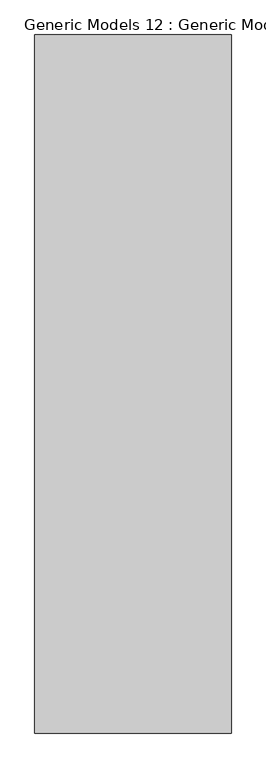
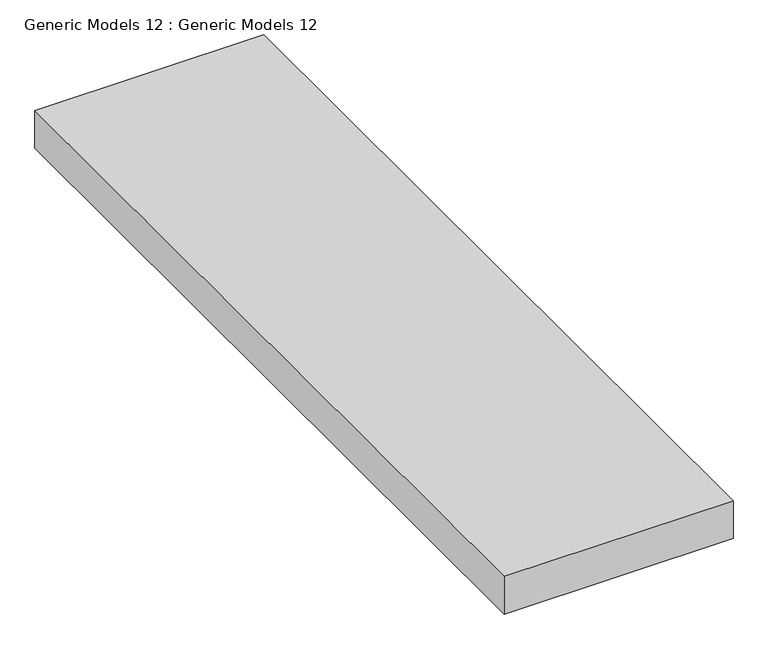
"""IFC4 building model written with IfcOpenShell, lengths in millimetres: proxy geometry, Generic Models 12 : Generic Models 12."""

from ifc_helpers import new_model, si_unit, frame, origin, place, context, project, spatial, polyline, outline, extrude, source, transform, mapped, element, save


def generic_models_12_generic_models_12_d8dec629(model_context):
    return source(origin(), model_context, "Body", "SweptSolid", [
        extrude(outline(polyline([(-8320.1161422, -4642.9842679), (-9196.4161422, -4642.9842679), (-9196.4161422, -1531.1171312), (-8320.1161422, -1531.1171312), (-8320.1161422, -4642.9842679)])), frame((0.0, 0.0, 5503.6617435), z_axis=(0.0, 0.0, 1.0), x_axis=(1.0, 0.0, 0.0)), (0.0, 0.0, 1.0), 152.4),
    ])


if __name__ == "__main__":
    model = new_model("IFC4")
    model_context = context("Model", 3, world=origin())
    ifc_project = project(units=[si_unit("LENGTHUNIT", "METRE", prefix="MILLI")], contexts=[model_context])
    site = spatial("IfcSite", under=ifc_project)
    building = spatial("IfcBuilding", under=site)
    placement = place(None, origin())
    generic_models_12_generic_models_12_shape = generic_models_12_generic_models_12_d8dec629(model_context)
    element("IfcBuildingElementProxy", 1, Name="Generic Models 12 : Generic Models 12", ObjectType="Generic Models 12 : Generic Models 12", at=placement, inside=building, context=model_context, shape_type="MappedRepresentation", body=[
        mapped(generic_models_12_generic_models_12_shape, transform((0.0, 0.0, 0.0), x_axis=(1.0, 0.0, 0.0), y_axis=(0.0, 1.0, 0.0), z_axis=(0.0, 0.0, 1.0))),
    ])
    save(model, "model.ifc")
